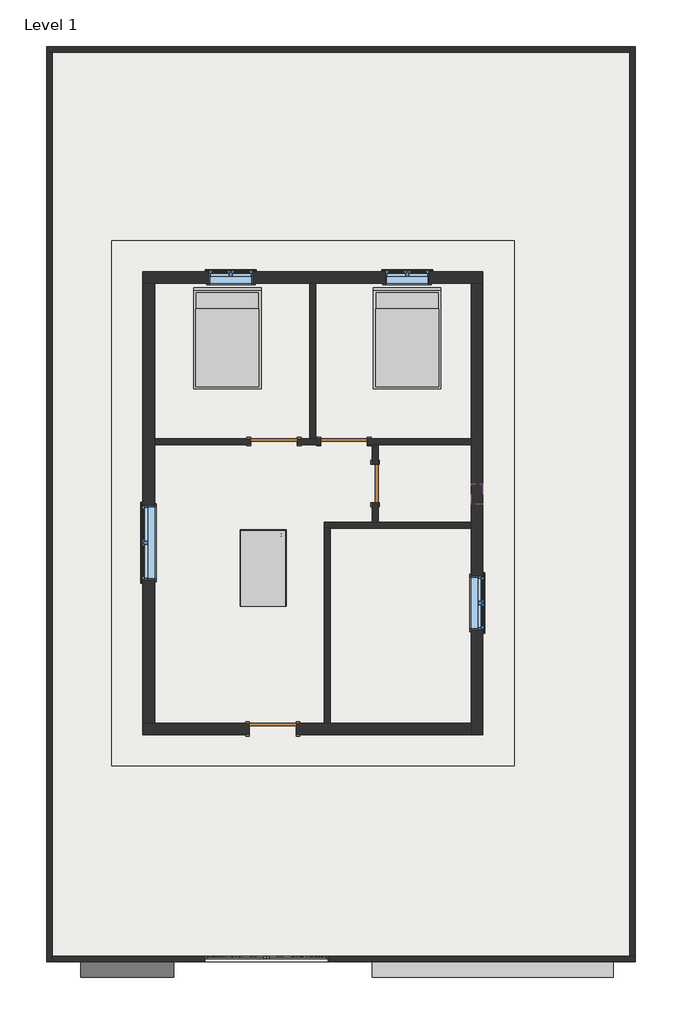
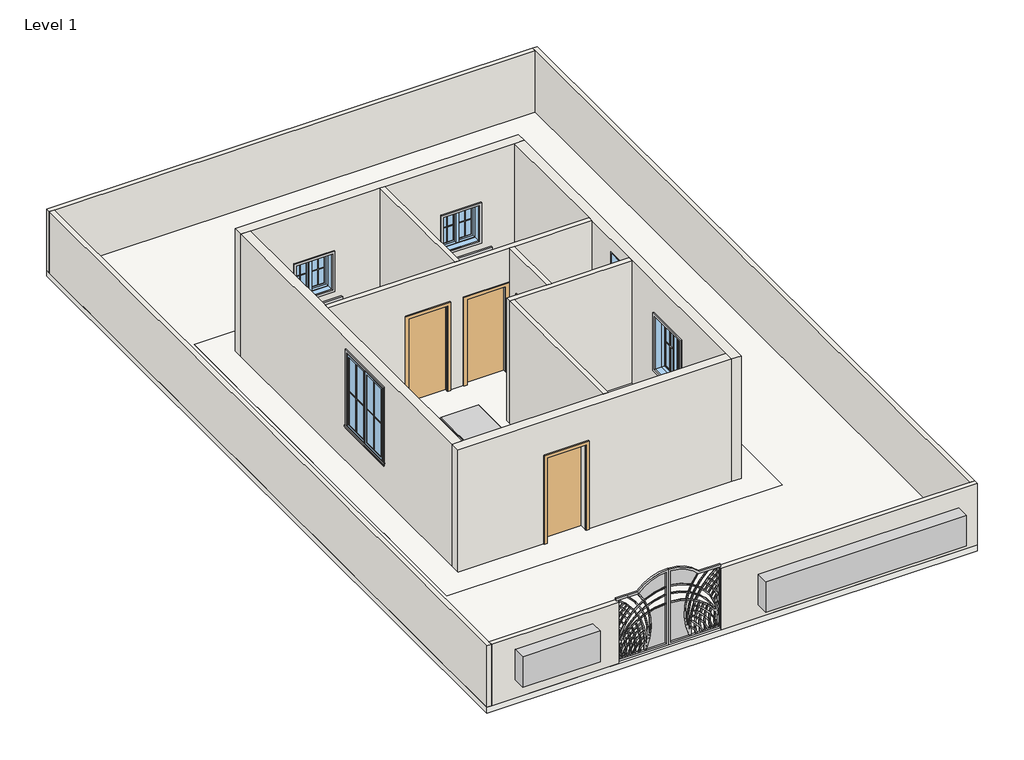
# One storey, incomplete: 18 proxies, 14 walls, 5 windows, 4 doors, 3 furniture elements, 2 slabs.
"""IFC4 building model written with IfcOpenShell, lengths in millimetres."""

from ifc_helpers import new_model, si_unit, frame, origin, origin_with_axes, place, context, project, spatial, polyline, outline, extrude, faceted_brep, transform, mapped, element, save
from components import generic_models_6bc30956, generic_models_2_generic_models_2_082925ae, muntin_pattern_2x2_muntin_pattern_2x2_b3fe6957, muntin_pattern_2x2_muntin_pattern_2x2_3e0ecaf2, muntin_pattern_2x2_muntin_pattern_2x2_bff912c5, muntin_pattern_2x2_muntin_pattern_2x2_c2194282, muntin_pattern_2x2_muntin_pattern_2x2_88bf7f41, muntin_pattern_2x2_muntin_pattern_2x2_3dfd0a47, trim_window_exterior_flat_with_sill_41619996, trim_window_exterior_flat_with_sill_e04b3088, trim_window_exterior_flat_with_sill_4930676f, trim_window_interior_flat_picture_frame_51c85655, trim_window_interior_flat_picture_frame_2a7685fe, trim_window_interior_flat_picture_frame_dd064338, door_f2b275c1, door_e5f9f3c4, door_305aa2a5, door_0ca8825f, bed_17739_bed_17739_15c61121, dining_table_14755_dining_table_14755_d89cb775, window_aa618e30, window_339605e1, window_c95ebb39, window_9ac97e1a

model = new_model("IFC4")

# Units and contexts
model_context = context("Model", 3, world=origin())
ifc_project = project(units=[si_unit("LENGTHUNIT", "METRE", prefix="MILLI")], contexts=[model_context])

# Site, building, storey
site = spatial("IfcSite", under=ifc_project)
building = spatial("IfcBuilding", under=site)
storey = spatial("IfcBuildingStorey", under=building, Name="Level 1", Elevation=0.0)

# Proxies
placement = place(None, origin())
generic_models_shape = generic_models_6bc30956(model_context)
element("IfcBuildingElementProxy", 1, Name="Generic Models", at=placement, inside=storey, context=model_context, shape_type="MappedRepresentation", body=[
    mapped(generic_models_shape, transform((-2169.6415084, -8339.9599223, 0.0), x_axis=(1.0, 0.0, 0.0), y_axis=(0.0, 1.0, 0.0), z_axis=(0.0, 0.0, 1.0))),
])
generic_models_2_generic_models_2_shape = generic_models_2_generic_models_2_082925ae(model_context)
element("IfcBuildingElementProxy", 2, Name="Generic Models 2 : Generic Models 2", ObjectType="Generic Models 2 : Generic Models 2", at=placement, inside=storey, context=model_context, shape_type="MappedRepresentation", body=[
    mapped(generic_models_2_generic_models_2_shape, transform((0.0, 0.0, 0.0), x_axis=(1.0, 0.0, 0.0), y_axis=(0.0, 1.0, 0.0), z_axis=(0.0, 0.0, 1.0))),
])
muntin_pattern_2x2_muntin_pattern_2x2_shape = muntin_pattern_2x2_muntin_pattern_2x2_b3fe6957(model_context)
element("IfcBuildingElementProxy", 3, Name="Muntin Pattern_2x2 : Muntin Pattern_2x2", ObjectType="Muntin Pattern_2x2 : Muntin Pattern_2x2", at=placement, inside=storey, context=model_context, shape_type="MappedRepresentation", body=[
    mapped(muntin_pattern_2x2_muntin_pattern_2x2_shape, transform((-3079.2790084, 5068.9185985, 984.25), x_axis=(1.0, 0.0, 0.0), y_axis=(0.0, 1.0, 0.0), z_axis=(0.0, 0.0, 1.0))),
])
element("IfcBuildingElementProxy", 4, Name="Muntin Pattern_2x2 : Muntin Pattern_2x2", ObjectType="Muntin Pattern_2x2 : Muntin Pattern_2x2", at=placement, inside=storey, context=model_context, shape_type="MappedRepresentation", body=[
    mapped(muntin_pattern_2x2_muntin_pattern_2x2_shape, transform((378.2959916, 5068.9185985, 984.25), x_axis=(1.0, 0.0, 0.0), y_axis=(0.0, 1.0, 0.0), z_axis=(0.0, 0.0, 1.0))),
])
muntin_pattern_2x2_muntin_pattern_2x2_2_shape = muntin_pattern_2x2_muntin_pattern_2x2_3e0ecaf2(model_context)
element("IfcBuildingElementProxy", 5, Name="Muntin Pattern_2x2 : Muntin Pattern_2x2", ObjectType="Muntin Pattern_2x2 : Muntin Pattern_2x2", at=placement, inside=storey, context=model_context, shape_type="MappedRepresentation", body=[
    mapped(muntin_pattern_2x2_muntin_pattern_2x2_2_shape, transform((-2650.6540084, 5068.9185985, 984.25), x_axis=(-1.0, 0.0, 0.0), y_axis=(0.0, -1.0, 0.0), z_axis=(0.0, 0.0, 1.0))),
])
element("IfcBuildingElementProxy", 6, Name="Muntin Pattern_2x2 : Muntin Pattern_2x2", ObjectType="Muntin Pattern_2x2 : Muntin Pattern_2x2", at=placement, inside=storey, context=model_context, shape_type="MappedRepresentation", body=[
    mapped(muntin_pattern_2x2_muntin_pattern_2x2_2_shape, transform((806.9209916, 5068.9185985, 984.25), x_axis=(-1.0, 0.0, 0.0), y_axis=(0.0, -1.0, 0.0), z_axis=(0.0, 0.0, 1.0))),
])
muntin_pattern_2x2_muntin_pattern_2x2_3_shape = muntin_pattern_2x2_muntin_pattern_2x2_bff912c5(model_context)
element("IfcBuildingElementProxy", 7, Name="Muntin Pattern_2x2 : Muntin Pattern_2x2", ObjectType="Muntin Pattern_2x2 : Muntin Pattern_2x2", at=placement, inside=storey, context=model_context, shape_type="MappedRepresentation", body=[
    mapped(muntin_pattern_2x2_muntin_pattern_2x2_3_shape, transform((-4579.4665084, -596.8689015, 984.25), x_axis=(0.0, 1.0, 0.0), y_axis=(-1.0, 0.0, 0.0), z_axis=(0.0, 0.0, 1.0))),
])
muntin_pattern_2x2_muntin_pattern_2x2_4_shape = muntin_pattern_2x2_muntin_pattern_2x2_c2194282(model_context)
element("IfcBuildingElementProxy", 8, Name="Muntin Pattern_2x2 : Muntin Pattern_2x2", ObjectType="Muntin Pattern_2x2 : Muntin Pattern_2x2", at=placement, inside=storey, context=model_context, shape_type="MappedRepresentation", body=[
    mapped(muntin_pattern_2x2_muntin_pattern_2x2_4_shape, transform((-4579.4665084, 123.8560985, 984.25), x_axis=(0.0, -1.0, 0.0), y_axis=(1.0, 0.0, 0.0), z_axis=(0.0, 0.0, 1.0))),
])
muntin_pattern_2x2_muntin_pattern_2x2_5_shape = muntin_pattern_2x2_muntin_pattern_2x2_88bf7f41(model_context)
element("IfcBuildingElementProxy", 9, Name="Muntin Pattern_2x2 : Muntin Pattern_2x2", ObjectType="Muntin Pattern_2x2 : Muntin Pattern_2x2", at=placement, inside=storey, context=model_context, shape_type="MappedRepresentation", body=[
    mapped(muntin_pattern_2x2_muntin_pattern_2x2_5_shape, transform((2068.9834916, -1158.8439015, 984.25), x_axis=(0.0, -1.0, 0.0), y_axis=(1.0, 0.0, 0.0), z_axis=(0.0, 0.0, 1.0))),
])
muntin_pattern_2x2_muntin_pattern_2x2_6_shape = muntin_pattern_2x2_muntin_pattern_2x2_3dfd0a47(model_context)
element("IfcBuildingElementProxy", 10, Name="Muntin Pattern_2x2 : Muntin Pattern_2x2", ObjectType="Muntin Pattern_2x2 : Muntin Pattern_2x2", at=placement, inside=storey, context=model_context, shape_type="MappedRepresentation", body=[
    mapped(muntin_pattern_2x2_muntin_pattern_2x2_6_shape, transform((2068.9834916, -1676.3689015, 984.25), x_axis=(0.0, 1.0, 0.0), y_axis=(-1.0, 0.0, 0.0), z_axis=(0.0, 0.0, 1.0))),
])
trim_window_exterior_flat_with_sill_shape = trim_window_exterior_flat_with_sill_41619996(model_context)
element("IfcBuildingElementProxy", 11, Name="Trim-Window-Exterior-Flat : with Sill", ObjectType="Trim-Window-Exterior-Flat : with Sill", at=placement, inside=storey, context=model_context, shape_type="MappedRepresentation", body=[
    mapped(trim_window_exterior_flat_with_sill_shape, transform((-2864.9665084, 5078.4435985, 1828.8), x_axis=(-1.0, 0.0, 0.0), y_axis=(0.0, 0.0, 1.0), z_axis=(0.0, 1.0, 0.0))),
])
element("IfcBuildingElementProxy", 12, Name="Trim-Window-Exterior-Flat : with Sill", ObjectType="Trim-Window-Exterior-Flat : with Sill", at=placement, inside=storey, context=model_context, shape_type="MappedRepresentation", body=[
    mapped(trim_window_exterior_flat_with_sill_shape, transform((592.6084916, 5078.4435985, 1828.8), x_axis=(-1.0, 0.0, 0.0), y_axis=(0.0, 0.0, 1.0), z_axis=(0.0, 1.0, 0.0))),
])
trim_window_exterior_flat_with_sill_2_shape = trim_window_exterior_flat_with_sill_e04b3088(model_context)
element("IfcBuildingElementProxy", 13, Name="Trim-Window-Exterior-Flat : with Sill", ObjectType="Trim-Window-Exterior-Flat : with Sill", at=placement, inside=storey, context=model_context, shape_type="MappedRepresentation", body=[
    mapped(trim_window_exterior_flat_with_sill_2_shape, transform((-4588.9915084, -236.5064015, 2743.2), x_axis=(0.0, -1.0, 0.0), y_axis=(0.0, 0.0, 1.0), z_axis=(-1.0, 0.0, 0.0))),
])
trim_window_exterior_flat_with_sill_3_shape = trim_window_exterior_flat_with_sill_4930676f(model_context)
element("IfcBuildingElementProxy", 14, Name="Trim-Window-Exterior-Flat : with Sill", ObjectType="Trim-Window-Exterior-Flat : with Sill", at=placement, inside=storey, context=model_context, shape_type="MappedRepresentation", body=[
    mapped(trim_window_exterior_flat_with_sill_3_shape, transform((2078.5084916, -1417.6064015, 2260.6), x_axis=(0.0, 1.0, 0.0), y_axis=(0.0, 0.0, 1.0), z_axis=(1.0, 0.0, 0.0))),
])
trim_window_interior_flat_picture_frame_shape = trim_window_interior_flat_picture_frame_51c85655(model_context)
element("IfcBuildingElementProxy", 15, Name="Trim-Window-Interior-Flat : Picture Frame", ObjectType="Trim-Window-Interior-Flat : Picture Frame", at=placement, inside=storey, context=model_context, shape_type="MappedRepresentation", body=[
    mapped(trim_window_interior_flat_picture_frame_shape, transform((-2864.9665084, 4849.8435985, 1828.8), x_axis=(1.0, 0.0, 0.0), y_axis=(0.0, 0.0, 1.0), z_axis=(0.0, -1.0, 0.0))),
])
element("IfcBuildingElementProxy", 16, Name="Trim-Window-Interior-Flat : Picture Frame", ObjectType="Trim-Window-Interior-Flat : Picture Frame", at=placement, inside=storey, context=model_context, shape_type="MappedRepresentation", body=[
    mapped(trim_window_interior_flat_picture_frame_shape, transform((592.6084916, 4849.8435985, 1828.8), x_axis=(1.0, 0.0, 0.0), y_axis=(0.0, 0.0, 1.0), z_axis=(0.0, -1.0, 0.0))),
])
trim_window_interior_flat_picture_frame_2_shape = trim_window_interior_flat_picture_frame_2a7685fe(model_context)
element("IfcBuildingElementProxy", 17, Name="Trim-Window-Interior-Flat : Picture Frame", ObjectType="Trim-Window-Interior-Flat : Picture Frame", at=placement, inside=storey, context=model_context, shape_type="MappedRepresentation", body=[
    mapped(trim_window_interior_flat_picture_frame_2_shape, transform((-4360.3915084, -236.5064015, 2743.2), x_axis=(0.0, 1.0, 0.0), y_axis=(0.0, 0.0, 1.0), z_axis=(1.0, 0.0, 0.0))),
])
trim_window_interior_flat_picture_frame_3_shape = trim_window_interior_flat_picture_frame_dd064338(model_context)
element("IfcBuildingElementProxy", 18, Name="Trim-Window-Interior-Flat : Picture Frame", ObjectType="Trim-Window-Interior-Flat : Picture Frame", at=placement, inside=storey, context=model_context, shape_type="MappedRepresentation", body=[
    mapped(trim_window_interior_flat_picture_frame_3_shape, transform((1849.9084916, -1417.6064015, 2260.6), x_axis=(0.0, -1.0, 0.0), y_axis=(0.0, 0.0, 1.0), z_axis=(-1.0, 0.0, 0.0))),
])

# Doors
door_shape = door_f2b275c1(model_context)
element("IfcDoor", 19, ObjectType="Single-Flush : 30\" x 80\"", at=placement, inside=storey, context=model_context, shape_type="MappedRepresentation", body=[
    mapped(door_shape, transform((-36.0415084, 925.5435985, 0.0), x_axis=(0.0, 1.0, 0.0), y_axis=(-1.0, 0.0, 0.0), z_axis=(0.0, 0.0, 1.0))),
])
door_2_shape = door_e5f9f3c4(model_context)
element("IfcDoor", 20, ObjectType="Single-Flush : 36\" x 84\"", at=placement, inside=storey, context=model_context, shape_type="MappedRepresentation", body=[
    mapped(door_2_shape, transform((-2017.2415084, 1744.6935985, 0.0), x_axis=(1.0, 0.0, 0.0), y_axis=(0.0, 1.0, 0.0), z_axis=(0.0, 0.0, 1.0))),
])
door_3_shape = door_305aa2a5(model_context)
element("IfcDoor", 21, ObjectType="Single-Flush : 36\" x 84\"", at=placement, inside=storey, context=model_context, shape_type="MappedRepresentation", body=[
    mapped(door_3_shape, transform((-645.6415084, 1744.6935985, 0.0), x_axis=(-1.0, 0.0, 0.0), y_axis=(0.0, -1.0, 0.0), z_axis=(0.0, 0.0, 1.0))),
])
door_4_shape = door_0ca8825f(model_context)
element("IfcDoor", 22, ObjectType="Single-Flush : 36\" x 84\"", at=placement, inside=storey, context=model_context, shape_type="MappedRepresentation", body=[
    mapped(door_4_shape, transform((-2042.6415084, -3887.7564015, 0.0), x_axis=(1.0, 0.0, 0.0), y_axis=(0.0, 1.0, 0.0), z_axis=(0.0, 0.0, 1.0))),
])

# Furniture
bed_17739_bed_17739_shape = bed_17739_bed_17739_15c61121(model_context)
element("IfcFurniture", 23, ObjectType="Bed_17739 : Bed_17739", at=placement, inside=storey, context=model_context, shape_type="MappedRepresentation", body=[
    mapped(bed_17739_bed_17739_shape, transform((-2931.6415084, 3744.9435985, 0.0), x_axis=(1.0, 0.0, 0.0), y_axis=(0.0, 1.0, 0.0), z_axis=(0.0, 0.0, 1.0))),
])
element("IfcFurniture", 24, ObjectType="Bed_17739 : Bed_17739", at=placement, inside=storey, context=model_context, shape_type="MappedRepresentation", body=[
    mapped(bed_17739_bed_17739_shape, transform((592.6084916, 3744.9435985, 0.0), x_axis=(1.0, 0.0, 0.0), y_axis=(0.0, 1.0, 0.0), z_axis=(0.0, 0.0, 1.0))),
])
dining_table_14755_dining_table_14755_shape = dining_table_14755_dining_table_14755_d89cb775(model_context)
element("IfcFurniture", 25, ObjectType="Dining_table_14755 : Dining_table_14755", at=placement, inside=storey, context=model_context, shape_type="MappedRepresentation", body=[
    mapped(dining_table_14755_dining_table_14755_shape, transform((-1781.6222109, -1485.4350296, 0.0), x_axis=(0.0, 1.0, 0.0), y_axis=(-1.0, 0.0, 0.0), z_axis=(0.0, 0.0, 1.0))),
])

# Slabs
element("IfcSlab", 26, ObjectType="Generic - 12\"", at=placement, inside=storey, context=model_context, shape_type="SweptSolid", body=[
    extrude(outline(polyline([(5067.1792532, 9490.8400777), (5067.1792532, -8454.2599223), (-6477.1207468, -8454.2599223), (-6477.1207468, 9490.8400777), (5067.1792532, 9490.8400777)])), frame((0.0, 0.0, -152.4), z_axis=(0.0, 0.0, 1.0), x_axis=(1.0, 0.0, 0.0)), (0.0, 0.0, 1.0), 152.4),
])
element("IfcSlab", 27, ObjectType="Generic - 12\"", at=placement, inside=storey, context=model_context, shape_type="SweptSolid", body=[
    extrude(outline(polyline([(2688.1084916, 5688.0435985), (2688.1084916, -4611.6564015), (-5198.5915084, -4611.6564015), (-5198.5915084, 5688.0435985), (2688.1084916, 5688.0435985)])), frame((0.0, 0.0, -152.4), z_axis=(0.0, 0.0, 1.0), x_axis=(1.0, 0.0, 0.0)), (0.0, 0.0, 1.0), 152.4),
])

# Walls
element("IfcWall", 28, ObjectType="WALL4.5\"", at=placement, inside=storey, context=model_context, shape_type="Brep", body=[
    faceted_brep([(-1560.0415084, 1687.5435985, 0.0), (-1102.8415084, 1687.5435985, 0.0), (-1102.8415084, 1687.5435985, 2133.6), (-188.4415084, 1687.5435985, 2133.6), (-188.4415084, 1687.5435985, 0.0), (-93.1915084, 1687.5435985, 0.0), (21.1084916, 1687.5435985, 0.0), (1849.9084916, 1687.5435985, 0.0), (1849.9084916, 1687.5435985, 3048.0), (21.1084916, 1687.5435985, 3048.0), (-93.1915084, 1687.5435985, 3048.0), (-4360.3915084, 1687.5435985, 3048.0), (-4360.3915084, 1687.5435985, 0.0), (-2474.4415084, 1687.5435985, 0.0), (-2474.4415084, 1687.5435985, 2133.6), (-1560.0415084, 1687.5435985, 2133.6), (-1102.8415084, 1801.8435985, 2133.6), (-1102.8415084, 1801.8435985, 0.0), (-1198.0915084, 1801.8435985, 0.0), (-1312.3915084, 1801.8435985, 0.0), (-1560.0415084, 1801.8435985, 0.0), (-1560.0415084, 1801.8435985, 2133.6), (-2474.4415084, 1801.8435985, 2133.6), (-2474.4415084, 1801.8435985, 0.0), (-4360.3915084, 1801.8435985, 0.0), (-4360.3915084, 1801.8435985, 3048.0), (-1312.3915084, 1801.8435985, 3048.0), (-1198.0915084, 1801.8435985, 3048.0), (1849.9084916, 1801.8435985, 3048.0), (1849.9084916, 1801.8435985, 0.0), (-188.4415084, 1801.8435985, 0.0), (-188.4415084, 1801.8435985, 2133.6)], [[[0, 1, 2, 3, 4, 5, 6, 7, 8, 9, 10, 11, 12, 13, 14, 15]], [[16, 17, 18, 19, 20, 21, 22, 23, 24, 25, 26, 27, 28, 29, 30, 31]], [[13, 12, 24, 23]], [[30, 29, 7, 6, 5, 4]], [[20, 19, 18, 17, 1, 0]], [[8, 7, 29, 28]], [[12, 11, 25, 24]], [[21, 20, 0, 15]], [[22, 21, 15, 14]], [[23, 22, 14, 13]], [[2, 1, 17, 16]], [[3, 2, 16, 31]], [[4, 3, 31, 30]], [[11, 10, 9, 8, 28, 27, 26, 25]]]),
])
element("IfcWall", 29, ObjectType="WALL4.5\"", at=placement, inside=storey, context=model_context, shape_type="SweptSolid", body=[
    extrude(outline(polyline([(-1312.3915084, 1801.8435985), (-1312.3915084, 4849.8435985), (-1198.0915084, 4849.8435985), (-1198.0915084, 1801.8435985), (-1312.3915084, 1801.8435985)])), origin_with_axes(), (0.0, 0.0, 1.0), 3048.0),
])
element("IfcWall", 30, ObjectType="WALL4.5\"", at=placement, inside=storey, context=model_context, shape_type="SweptSolid", body=[
    extrude(outline(polyline([(1687.5435985, 0.0), (1306.5435985, 0.0), (1306.5435985, 2032.0), (544.5435985, 2032.0), (544.5435985, 0.0), (163.5435985, 0.0), (163.5435985, 3048.0), (1687.5435985, 3048.0), (1687.5435985, 0.0)])), frame((-93.1915084, 0.0, 0.0), z_axis=(1.0, 0.0, 0.0), x_axis=(0.0, 1.0, 0.0)), (0.0, 0.0, 1.0), 114.3),
])
element("IfcWall", 31, ObjectType="WALL4.5\"", at=placement, inside=storey, context=model_context, shape_type="Brep", body=[
    faceted_brep([(1849.9084916, 163.5435985, 0.0), (21.1084916, 163.5435985, 0.0), (-93.1915084, 163.5435985, 0.0), (-1032.9915084, 163.5435985, 0.0), (-1032.9915084, 163.5435985, 3048.0), (-93.1915084, 163.5435985, 3048.0), (21.1084916, 163.5435985, 3048.0), (1849.9084916, 163.5435985, 3048.0), (1849.9084916, 49.2435985, 0.0), (1849.9084916, 49.2435985, 3048.0), (-918.6915084, 49.2435985, 3048.0), (-1032.9915084, 49.2435985, 3048.0), (-1032.9915084, 49.2435985, 0.0), (-918.6915084, 49.2435985, 0.0)], [[[0, 1, 2, 3, 4, 5, 6, 7]], [[8, 9, 10, 11, 12, 13]], [[3, 2, 1, 0, 8, 13, 12]], [[0, 7, 9, 8]], [[4, 3, 12, 11]], [[7, 6, 5, 4, 11, 10, 9]]]),
])
element("IfcWall", 32, ObjectType="WALL4.5\"", at=placement, inside=storey, context=model_context, shape_type="SweptSolid", body=[
    extrude(outline(polyline([(-1032.9915084, -3773.4564015), (-1032.9915084, 49.2435985), (-918.6915084, 49.2435985), (-918.6915084, -3773.4564015), (-1032.9915084, -3773.4564015)])), origin_with_axes(), (0.0, 0.0, 1.0), 3048.0),
])
element("IfcWall", 33, ObjectType="WALL4.5\"", at=placement, inside=storey, context=model_context, shape_type="Brep", body=[
    faceted_brep([(-6477.1207468, 9376.5400777, 0.0), (-6362.8207468, 9376.5400777, 0.0), (4952.8792532, 9376.5400777, 0.0), (4952.8792532, 9376.5400777, 1524.0), (-6362.8207468, 9376.5400777, 1524.0), (-6477.1207468, 9376.5400777, 1524.0), (-6477.1207468, 9490.8400777, 0.0), (-6477.1207468, 9490.8400777, 1524.0), (4952.8792532, 9490.8400777, 1524.0), (4952.8792532, 9490.8400777, 0.0)], [[[0, 1, 2, 3, 4, 5]], [[6, 7, 8, 9]], [[2, 1, 0, 6, 9]], [[5, 4, 3, 8, 7]], [[0, 5, 7, 6]], [[3, 2, 9, 8]]]),
])
element("IfcWall", 34, ObjectType="WALL4.5\"", at=placement, inside=storey, context=model_context, shape_type="Brep", body=[
    faceted_brep([(-6362.8207468, -8454.2599223, 0.0), (-6362.8207468, -8339.9599223, 0.0), (-6362.8207468, 9376.5400777, 0.0), (-6362.8207468, 9376.5400777, 1524.0), (-6362.8207468, -8339.9599223, 1524.0), (-6362.8207468, -8454.2599223, 1524.0), (-6477.1207468, -8454.2599223, 0.0), (-6477.1207468, -8454.2599223, 1524.0), (-6477.1207468, 9376.5400777, 1524.0), (-6477.1207468, 9376.5400777, 0.0)], [[[0, 1, 2, 3, 4, 5]], [[6, 7, 8, 9]], [[2, 1, 0, 6, 9]], [[5, 4, 3, 8, 7]], [[0, 5, 7, 6]], [[3, 2, 9, 8]]]),
])
element("IfcWall", 35, ObjectType="WALL4.5\"", at=placement, inside=storey, context=model_context, shape_type="Brep", body=[
    faceted_brep([(5067.1792532, -8339.9599223, 0.0), (4952.8792532, -8339.9599223, 0.0), (-958.9707468, -8339.9599223, 0.0), (-958.9707468, -8339.9599223, 1524.0), (4952.8792532, -8339.9599223, 1524.0), (5067.1792532, -8339.9599223, 1524.0), (5067.1792532, -8454.2599223, 0.0), (5067.1792532, -8454.2599223, 1524.0), (-958.9707468, -8454.2599223, 1524.0), (-958.9707468, -8454.2599223, 0.0)], [[[0, 1, 2, 3, 4, 5]], [[6, 7, 8, 9]], [[2, 1, 0, 6, 9]], [[3, 2, 9, 8]], [[5, 4, 3, 8, 7]], [[0, 5, 7, 6]]]),
])
element("IfcWall", 36, ObjectType="WALL4.5\"", at=placement, inside=storey, context=model_context, shape_type="Brep", body=[
    faceted_brep([(4952.8792532, 9490.8400777, 0.0), (4952.8792532, 9376.5400777, 0.0), (4952.8792532, -8339.9599223, 0.0), (4952.8792532, -8339.9599223, 1524.0), (4952.8792532, 9376.5400777, 1524.0), (4952.8792532, 9490.8400777, 1524.0), (5067.1792532, 9490.8400777, 0.0), (5067.1792532, 9490.8400777, 1524.0), (5067.1792532, -8339.9599223, 1524.0), (5067.1792532, -8339.9599223, 0.0)], [[[0, 1, 2, 3, 4, 5]], [[6, 7, 8, 9]], [[2, 1, 0, 6, 9]], [[5, 4, 3, 8, 7]], [[0, 5, 7, 6]], [[3, 2, 9, 8]]]),
])
element("IfcWall", 37, ObjectType="WALL4.5\"", at=placement, inside=storey, context=model_context, shape_type="SweptSolid", body=[
    extrude(outline(polyline([(-6362.8207468, -8339.9599223), (-3371.9707468, -8339.9599223), (-3371.9707468, -8454.2599223), (-6362.8207468, -8454.2599223), (-6362.8207468, -8339.9599223)])), origin_with_axes(), (0.0, 0.0, 1.0), 1524.0),
])
element("IfcWall", 38, ObjectType="WALL9\"", at=placement, inside=storey, context=model_context, shape_type="Brep", body=[
    faceted_brep([(-4588.9915084, 4849.8435985, 0.0), (-4360.3915084, 4849.8435985, 0.0), (-1312.3915084, 4849.8435985, 0.0), (-1198.0915084, 4849.8435985, 0.0), (1849.9084916, 4849.8435985, 0.0), (2078.5084916, 4849.8435985, 0.0), (2078.5084916, 4849.8435985, 3048.0), (1849.9084916, 4849.8435985, 3048.0), (-1198.0915084, 4849.8435985, 3048.0), (-1312.3915084, 4849.8435985, 3048.0), (-4360.3915084, 4849.8435985, 3048.0), (-4588.9915084, 4849.8435985, 3048.0), (-2433.1665084, 4849.8435985, 1828.8), (-2433.1665084, 4849.8435985, 914.4), (-3296.7665084, 4849.8435985, 914.4), (-3296.7665084, 4849.8435985, 1828.8), (1024.4084916, 4849.8435985, 1828.8), (1024.4084916, 4849.8435985, 914.4), (160.8084916, 4849.8435985, 914.4), (160.8084916, 4849.8435985, 1828.8), (-4588.9915084, 5078.4435985, 0.0), (-4588.9915084, 5078.4435985, 3048.0), (2078.5084916, 5078.4435985, 3048.0), (2078.5084916, 5078.4435985, 0.0), (-2433.1665084, 5078.4435985, 1828.8), (-3296.7665084, 5078.4435985, 1828.8), (-3296.7665084, 5078.4435985, 914.4), (-2433.1665084, 5078.4435985, 914.4), (1024.4084916, 5078.4435985, 1828.8), (160.8084916, 5078.4435985, 1828.8), (160.8084916, 5078.4435985, 914.4), (1024.4084916, 5078.4435985, 914.4)], [[[0, 1, 2, 3, 4, 5, 6, 7, 8, 9, 10, 11], [12, 13, 14, 15], [16, 17, 18, 19]], [[20, 21, 22, 23], [24, 25, 26, 27], [28, 29, 30, 31]], [[5, 4, 3, 2, 1, 0, 20, 23]], [[6, 5, 23, 22]], [[0, 11, 21, 20]], [[13, 12, 24, 27]], [[14, 13, 27, 26]], [[15, 14, 26, 25]], [[12, 15, 25, 24]], [[17, 16, 28, 31]], [[18, 17, 31, 30]], [[19, 18, 30, 29]], [[16, 19, 29, 28]], [[11, 10, 9, 8, 7, 6, 22, 21]]]),
])
element("IfcWall", 39, ObjectType="WALL9\"", at=placement, inside=storey, context=model_context, shape_type="Brep", body=[
    faceted_brep([(1849.9084916, 4849.8435985, 0.0), (1849.9084916, 1801.8435985, 0.0), (1849.9084916, 1687.5435985, 0.0), (1849.9084916, 163.5435985, 0.0), (1849.9084916, 49.2435985, 0.0), (1849.9084916, -3773.4564015, 0.0), (1849.9084916, -4002.0564015, 0.0), (1849.9084916, -4002.0564015, 3048.0), (1849.9084916, -3773.4564015, 3048.0), (1849.9084916, 49.2435985, 3048.0), (1849.9084916, 163.5435985, 3048.0), (1849.9084916, 1687.5435985, 3048.0), (1849.9084916, 1801.8435985, 3048.0), (1849.9084916, 4849.8435985, 3048.0), (1849.9084916, -1938.3064015, 2260.6), (1849.9084916, -1938.3064015, 914.4), (1849.9084916, -896.9064015, 914.4), (1849.9084916, -896.9064015, 2260.6), (1849.9084916, 512.7935985, 2743.2), (1849.9084916, 512.7935985, 2133.6), (1849.9084916, 919.1935985, 2133.6), (1849.9084916, 919.1935985, 2743.2), (2078.5084916, 4849.8435985, 0.0), (2078.5084916, 4849.8435985, 3048.0), (2078.5084916, -4002.0564015, 3048.0), (2078.5084916, -4002.0564015, 0.0), (2078.5084916, -1938.3064015, 2260.6), (2078.5084916, -896.9064015, 2260.6), (2078.5084916, -896.9064015, 914.4), (2078.5084916, -1938.3064015, 914.4), (2078.5084916, 512.7935985, 2743.2), (2078.5084916, 919.1935985, 2743.2), (2078.5084916, 919.1935985, 2133.6), (2078.5084916, 512.7935985, 2133.6)], [[[0, 1, 2, 3, 4, 5, 6, 7, 8, 9, 10, 11, 12, 13], [14, 15, 16, 17], [18, 19, 20, 21]], [[22, 23, 24, 25], [26, 27, 28, 29], [30, 31, 32, 33]], [[6, 5, 4, 3, 2, 1, 0, 22, 25]], [[0, 13, 23, 22]], [[7, 6, 25, 24]], [[15, 14, 26, 29]], [[16, 15, 29, 28]], [[17, 16, 28, 27]], [[14, 17, 27, 26]], [[19, 18, 30, 33]], [[20, 19, 33, 32]], [[21, 20, 32, 31]], [[18, 21, 31, 30]], [[13, 12, 11, 10, 9, 8, 7, 24, 23]]]),
])
element("IfcWall", 40, ObjectType="WALL9\"", at=placement, inside=storey, context=model_context, shape_type="Brep", body=[
    faceted_brep([(1849.9084916, -3773.4564015, 0.0), (-918.6915084, -3773.4564015, 0.0), (-1032.9915084, -3773.4564015, 0.0), (-1585.4415084, -3773.4564015, 0.0), (-1585.4415084, -3773.4564015, 2133.6), (-2499.8415084, -3773.4564015, 2133.6), (-2499.8415084, -3773.4564015, 0.0), (-4360.3915084, -3773.4564015, 0.0), (-4588.9915084, -3773.4564015, 0.0), (-4588.9915084, -3773.4564015, 3048.0), (-4360.3915084, -3773.4564015, 3048.0), (-1032.9915084, -3773.4564015, 3048.0), (-918.6915084, -3773.4564015, 3048.0), (1849.9084916, -3773.4564015, 3048.0), (-1585.4415084, -4002.0564015, 2133.6), (-1585.4415084, -4002.0564015, 0.0), (1849.9084916, -4002.0564015, 0.0), (1849.9084916, -4002.0564015, 3048.0), (-4588.9915084, -4002.0564015, 3048.0), (-4588.9915084, -4002.0564015, 0.0), (-2499.8415084, -4002.0564015, 0.0), (-2499.8415084, -4002.0564015, 2133.6)], [[[0, 1, 2, 3, 4, 5, 6, 7, 8, 9, 10, 11, 12, 13]], [[14, 15, 16, 17, 18, 19, 20, 21]], [[20, 19, 8, 7, 6]], [[16, 15, 3, 2, 1, 0]], [[0, 13, 17, 16]], [[9, 8, 19, 18]], [[4, 3, 15, 14]], [[5, 4, 14, 21]], [[6, 5, 21, 20]], [[13, 12, 11, 10, 9, 18, 17]]]),
])
element("IfcWall", 41, ObjectType="WALL9\"", at=placement, inside=storey, context=model_context, shape_type="Brep", body=[
    faceted_brep([(-4360.3915084, -3773.4564015, 0.0), (-4360.3915084, 1687.5435985, 0.0), (-4360.3915084, 1801.8435985, 0.0), (-4360.3915084, 4849.8435985, 0.0), (-4360.3915084, 4849.8435985, 3048.0), (-4360.3915084, 1801.8435985, 3048.0), (-4360.3915084, 1687.5435985, 3048.0), (-4360.3915084, -3773.4564015, 3048.0), (-4360.3915084, 487.3935985, 2743.2), (-4360.3915084, 487.3935985, 914.4), (-4360.3915084, -960.4064015, 914.4), (-4360.3915084, -960.4064015, 2743.2), (-4588.9915084, -3773.4564015, 0.0), (-4588.9915084, -3773.4564015, 3048.0), (-4588.9915084, 4849.8435985, 3048.0), (-4588.9915084, 4849.8435985, 0.0), (-4588.9915084, 487.3935985, 2743.2), (-4588.9915084, -960.4064015, 2743.2), (-4588.9915084, -960.4064015, 914.4), (-4588.9915084, 487.3935985, 914.4)], [[[0, 1, 2, 3, 4, 5, 6, 7], [8, 9, 10, 11]], [[12, 13, 14, 15], [16, 17, 18, 19]], [[3, 2, 1, 0, 12, 15]], [[0, 7, 13, 12]], [[4, 3, 15, 14]], [[9, 8, 16, 19]], [[10, 9, 19, 18]], [[11, 10, 18, 17]], [[8, 11, 17, 16]], [[7, 6, 5, 4, 14, 13]]]),
])

# Windows
window_shape = window_aa618e30(model_context)
element("IfcWindow", 42, ObjectType="Fixed : 16\" x 24\"", at=placement, inside=storey, context=model_context, shape_type="MappedRepresentation", body=[
    mapped(window_shape, transform((1964.2084916, 677.8935985, 1219.2), x_axis=(0.0, -1.0, 0.0), y_axis=(1.0, 0.0, 0.0), z_axis=(0.0, 0.0, 1.0))),
])
window_2_shape = window_339605e1(model_context)
element("IfcWindow", 43, ObjectType="Window-Casement-Double : 34\" x 36\"", at=placement, inside=storey, context=model_context, shape_type="MappedRepresentation", body=[
    mapped(window_2_shape, transform((-2864.9665084, 4964.1435985, 0.0), x_axis=(1.0, 0.0, 0.0), y_axis=(0.0, 1.0, 0.0), z_axis=(0.0, 0.0, 1.0))),
])
element("IfcWindow", 44, ObjectType="Window-Casement-Double : 34\" x 36\"", at=placement, inside=storey, context=model_context, shape_type="MappedRepresentation", body=[
    mapped(window_2_shape, transform((592.6084916, 4964.1435985, 0.0), x_axis=(1.0, 0.0, 0.0), y_axis=(0.0, 1.0, 0.0), z_axis=(0.0, 0.0, 1.0))),
])
window_3_shape = window_c95ebb39(model_context)
element("IfcWindow", 45, ObjectType="Window-Casement-Double : 41\" x 53\"", at=placement, inside=storey, context=model_context, shape_type="MappedRepresentation", body=[
    mapped(window_3_shape, transform((1964.2084916, -1417.6064015, 0.0), x_axis=(0.0, -1.0, 0.0), y_axis=(1.0, 0.0, 0.0), z_axis=(0.0, 0.0, 1.0))),
])
window_4_shape = window_9ac97e1a(model_context)
element("IfcWindow", 46, ObjectType="Window-Casement-Double : 57\" x 72\"", at=placement, inside=storey, context=model_context, shape_type="MappedRepresentation", body=[
    mapped(window_4_shape, transform((-4474.6915084, -236.5064015, 0.0), x_axis=(0.0, 1.0, 0.0), y_axis=(-1.0, 0.0, 0.0), z_axis=(0.0, 0.0, 1.0))),
])

save(model, "model.ifc")

# Revit data of these elements
# Type
#   m.s. sheet = none
#   2" x2" pipe = none
#   1"x1"pipe = none
#   Default Elevation = 0
# Type "Muntin Pattern_2x2 : Muntin Pattern_2x2"
#   Width [instance default] = 4' - 0"
#   Thickness = 0' - 0 1/2"
#   Height [instance default] = 4' - 0"
#   Distance = 0' - 0 3/4"
#   Interior Material [instance default] = none
#   Exterior Material [instance default] = none
#   Default Elevation = 0
# Type "Trim-Window-Exterior-Flat : with Sill"
#   Trim Width = 0' - 2 1/4"
#   Trim Thickness_Picture Frame = 0' - 1 1/4"
#   Trim Thickness_with Sill = 0' - 0 3/4"
#   Sill Thickness = 0' - 1 1/4"
#   Opening Width [instance default] = 2' - 0"
#   Opening Height [instance default] = 3' - 0"
#   Default Elevation = 4' - 0"
#   Sill = yes
#   Picture Frame = no
#   Trim Material [instance default] = none
# Type "Trim-Window-Interior-Flat : Picture Frame"
#   Trim Thickness_Picture Frame = 0' - 1 1/4"
#   Trim Width = 0' - 2 1/4"
#   Trim Thickness_with Sill = 0' - 0 3/4"
#   Sill Thickness = 0' - 1 1/4"
#   Opening Width [instance default] = 2' - 0"
#   Opening Height [instance default] = 3' - 0"
#   Default Elevation = 4' - 0"
#   Sill = no
#   Picture Frame = yes
#   Trim Material [instance default] = none
# Type "Single-Flush : 30\" x 80\""
#   Type Mark = "5"
#   Construction Type Id = "MDOOR"
#   Assembly Code = "C1020"
#   Analytic Construction = "Metal"
#   Thickness = 0' - 2"
#   Heat Transfer Coefficient (U) = 0.651978 BTU/(h·ft²·°F)
#   Height = 6' - 8"
#   Trim Projection Ext = 0' - 1"
#   Trim Projection Int = 0' - 1"
#   Trim Width = 0' - 3"
#   Width = 2' - 6"
#   Define Thermal Properties by = 1
#   Define Thermal Properties by = 1
#   Door Material = Door - Panel
#   Frame Material = Door - Frame
#   Visual Light Transmittance = 0
#   Solar Heat Gain Coefficient = 0
#   Function = (empty or 0)
#   Wall Closure = (empty or 0)
# Type "Single-Flush : 36\" x 84\""
#   Type Mark = "1"
#   Construction Type Id = "MDOOR"
#   Assembly Code = "C1020"
#   Analytic Construction = "Metal"
#   Thickness = 0' - 2"
#   Heat Transfer Coefficient (U) = 0.651978 BTU/(h·ft²·°F)
#   Height = 7' - 0"
#   Trim Projection Ext = 0' - 1"
#   Trim Projection Int = 0' - 1"
#   Trim Width = 0' - 3"
#   Width = 3' - 0"
#   Define Thermal Properties by = 1
#   Define Thermal Properties by = 1
#   Door Material = Door - Panel
#   Frame Material = Door - Frame
#   Visual Light Transmittance = 0
#   Solar Heat Gain Coefficient = 0
#   Function = (empty or 0)
#   Wall Closure = (empty or 0)
# Type "Bed_17739 : Bed_17739"
#   Default Elevation = 0
# Type "Dining_table_14755 : Dining_table_14755"
#   Lengte [instance default] = 4' - 11.05512"
#   Breedte [instance default] = 2' - 11.43307"
#   Tafelblad = none
#   Poten = none
#   Default Elevation = 0
# Type "Generic - 12\""
#   Assembly Code = "B1010"
#   Function = 0
#   Layers, outside or top first: 0' - 6" no material (function 1)
# Type "WALL4.5\""
#   Assembly Code = "B2010"
#   Layers, outside or top first: 0' - 4 1/2" no material (function 1)
# Type "WALL9\""
#   Assembly Code = "B2010"
#   Layers, outside or top first: 0' - 9" no material (function 1)
# Type "Fixed : 16\" x 24\""
#   Type Mark = "4"
#   Construction Type Id = "GSP4R"
#   Assembly Code = "B2020100"
#   Analytic Construction = "1/8 in Pilkington single glazing"
#   Visual Light Transmittance = 0.9
#   Solar Heat Gain Coefficient = 0.78
#   Heat Transfer Coefficient (U) = 0.6496 BTU/(h·ft²·°F)
#   Height = 2' - 0"
#   Default Sill Height = 3' - 0"
#   Width = 1' - 4"
#   Window Inset = 0' - 0 3/4"
#   Define Thermal Properties by = 1
#   Define Thermal Properties by = 1
#   Glass Pane Material = Glass
#   Sash Material = Sash
#   Wall Closure = (empty or 0)
# Type "Window-Casement-Double : 34\" x 36\""
#   Type Mark = "14"
#   Fire Rating = "0.5h"
#   Assembly Code = "B2020100"
#   Analytic Construction = "Double glazing - domestic"
#   Frame Extension [instance default] = 0' - 0 1/4"
#   Window Inset [instance default] = 0' - 0"
#   Wall Thickness [instance default] = 0' - 6"
#   Interior Wall Closure [instance default] = 0' - 2 1/4"
#   Half Width = 1' - 5"
#   Visual Light Transmittance = 0.81
#   Thermal Resistance (R) = 1.8146 (h·ft²·°F)/BTU
#   Solar Heat Gain Coefficient = 0.76
#   Rough Width = 2' - 10 1/2"
#   Rough Height = 3' - 0 1/2"
#   Height = 3' - 0"
#   Heat Transfer Coefficient (U) = 0.5511 BTU/(h·ft²·°F)
#   Exterior Wall Closure [instance default] = 0' - 1 1/4"
#   Extension Jamb [instance default] = 0' - 2 1/4"
#   Default Sill Height = 3' - 0"
#   Width = 2' - 10"
#   Define Thermal Properties by = 0
#   Muntin Visibility = yes
#   Interior Trim Visibility [instance default] = yes
#   Exterior Trim Visibility [instance default] = yes
#   Extension Jamb Visibility [instance default] = yes
#   Interior Trim Material = Wood - Stained
#   Muntin Pattern = Muntin Pattern_2x2 : Muntin Pattern_2x2
#   Interior Trim = Trim-Window-Interior-Flat : Picture Frame
#   Interior Frame Material = Wood - Stained
#   Glass Panel Material = Glass
#   Exterior Trim Material = Clad - White
#   Exterior Trim = Trim-Window-Exterior-Flat : with Sill
#   Exterior Frame Material = Clad - White
#   Wall Closure = (empty or 0)
# Type "Window-Casement-Double : 41\" x 53\""
#   Type Mark = "15"
#   Fire Rating = "0.5h"
#   Assembly Code = "B2020100"
#   Analytic Construction = "Double glazing - domestic"
#   Frame Extension [instance default] = 0' - 0 1/4"
#   Window Inset [instance default] = 0' - 0"
#   Wall Thickness [instance default] = 0' - 6"
#   Interior Wall Closure [instance default] = 0' - 2 1/4"
#   Half Width = 1' - 8 1/2"
#   Visual Light Transmittance = 0.81
#   Thermal Resistance (R) = 1.8146 (h·ft²·°F)/BTU
#   Solar Heat Gain Coefficient = 0.76
#   Rough Width = 3' - 5 1/2"
#   Rough Height = 4' - 5 1/2"
#   Height = 4' - 5"
#   Heat Transfer Coefficient (U) = 0.5511 BTU/(h·ft²·°F)
#   Exterior Wall Closure [instance default] = 0' - 1 1/4"
#   Extension Jamb [instance default] = 0' - 2 1/4"
#   Default Sill Height = 3' - 0"
#   Width = 3' - 5"
#   Define Thermal Properties by = 0
#   Muntin Visibility = yes
#   Interior Trim Visibility [instance default] = yes
#   Exterior Trim Visibility [instance default] = yes
#   Extension Jamb Visibility [instance default] = yes
#   Interior Trim Material = Wood - Stained
#   Muntin Pattern = Muntin Pattern_2x2 : Muntin Pattern_2x2
#   Interior Trim = Trim-Window-Interior-Flat : Picture Frame
#   Interior Frame Material = Wood - Stained
#   Glass Panel Material = Glass
#   Exterior Trim Material = Clad - White
#   Exterior Trim = Trim-Window-Exterior-Flat : with Sill
#   Exterior Frame Material = Clad - White
#   Wall Closure = (empty or 0)
# Type "Window-Casement-Double : 57\" x 72\""
#   Type Mark = "17"
#   Fire Rating = "0.5h"
#   Assembly Code = "B2020100"
#   Analytic Construction = "Double glazing - domestic"
#   Frame Extension [instance default] = 0' - 0 1/4"
#   Window Inset [instance default] = 0' - 0"
#   Wall Thickness [instance default] = 0' - 6"
#   Interior Wall Closure [instance default] = 0' - 2 1/4"
#   Half Width = 2' - 4 1/2"
#   Visual Light Transmittance = 0.81
#   Thermal Resistance (R) = 1.8146 (h·ft²·°F)/BTU
#   Solar Heat Gain Coefficient = 0.76
#   Rough Width = 4' - 9 1/2"
#   Rough Height = 6' - 0 1/2"
#   Height = 6' - 0"
#   Heat Transfer Coefficient (U) = 0.5511 BTU/(h·ft²·°F)
#   Exterior Wall Closure [instance default] = 0' - 1 1/4"
#   Extension Jamb [instance default] = 0' - 2 1/4"
#   Default Sill Height = 3' - 0"
#   Width = 4' - 9"
#   Define Thermal Properties by = 0
#   Muntin Visibility = yes
#   Interior Trim Visibility [instance default] = yes
#   Exterior Trim Visibility [instance default] = yes
#   Extension Jamb Visibility [instance default] = yes
#   Interior Trim Material = Wood - Stained
#   Muntin Pattern = Muntin Pattern_2x2 : Muntin Pattern_2x2
#   Interior Trim = Trim-Window-Interior-Flat : Picture Frame
#   Interior Frame Material = Wood - Stained
#   Glass Panel Material = Glass
#   Exterior Trim Material = Clad - White
#   Exterior Trim = Trim-Window-Exterior-Flat : with Sill
#   Exterior Frame Material = Clad - White
#   Wall Closure = (empty or 0)
# Element 1 (IfcBuildingElementProxy)
#   Phase Created = New Construction
#   Materials on its faces: "r1"
# Element 2 (IfcBuildingElementProxy, "Generic Models 2 : Generic Models 2")
#   Phase Created = New Construction
#   Materials on its faces: "Carpet (1)"
# Elements 3, 4, 5, 6 (IfcBuildingElementProxy, "Muntin Pattern_2x2 : Muntin Pattern_2x2")
#   Width = 0' - 11 5/8"
#   Height = 2' - 6 1/2"
#   Interior Material = Wood - Stained
#   Exterior Material = Clad - White
#   Phase Created = New Construction
#   Materials on its faces: "Clad - White", "Wood - Stained"
# Elements 7, 8 (IfcBuildingElementProxy, "Muntin Pattern_2x2 : Muntin Pattern_2x2")
#   Width = 1' - 11 1/8"
#   Height = 5' - 6 1/2"
#   Interior Material = Wood - Stained
#   Exterior Material = Clad - White
#   Phase Created = New Construction
#   Materials on its faces: "Clad - White", "Wood - Stained"
# Elements 9, 10 (IfcBuildingElementProxy, "Muntin Pattern_2x2 : Muntin Pattern_2x2")
#   Width = 1' - 3 1/8"
#   Height = 3' - 11 1/2"
#   Interior Material = Wood - Stained
#   Exterior Material = Clad - White
#   Phase Created = New Construction
#   Materials on its faces: "Clad - White", "Wood - Stained"
# Elements 11, 12 (IfcBuildingElementProxy, "Trim-Window-Exterior-Flat : with Sill")
#   Opening Width = 2' - 10"
#   Opening Height = 3' - 0"
#   Trim Material = Clad - White
#   Phase Created = New Construction
#   Materials on its faces: "Clad - White"
# Element 13 (IfcBuildingElementProxy, "Trim-Window-Exterior-Flat : with Sill")
#   Opening Width = 4' - 9"
#   Opening Height = 6' - 0"
#   Trim Material = Clad - White
#   Phase Created = New Construction
#   Materials on its faces: "Clad - White"
# Element 14 (IfcBuildingElementProxy, "Trim-Window-Exterior-Flat : with Sill")
#   Opening Width = 3' - 5"
#   Opening Height = 4' - 5"
#   Trim Material = Clad - White
#   Phase Created = New Construction
#   Materials on its faces: "Clad - White"
# Elements 15, 16 (IfcBuildingElementProxy, "Trim-Window-Interior-Flat : Picture Frame")
#   Opening Width = 2' - 10"
#   Opening Height = 3' - 0"
#   Trim Material = Wood - Stained
#   Phase Created = New Construction
#   Materials on its faces: "Wood - Stained"
# Element 17 (IfcBuildingElementProxy, "Trim-Window-Interior-Flat : Picture Frame")
#   Opening Width = 4' - 9"
#   Opening Height = 6' - 0"
#   Trim Material = Wood - Stained
#   Phase Created = New Construction
#   Materials on its faces: "Wood - Stained"
# Element 18 (IfcBuildingElementProxy, "Trim-Window-Interior-Flat : Picture Frame")
#   Opening Width = 3' - 5"
#   Opening Height = 4' - 5"
#   Trim Material = Wood - Stained
#   Phase Created = New Construction
#   Materials on its faces: "Wood - Stained"
# Element 19 (IfcDoor, "Single-Flush : 30\" x 80\"")
#   Phase Created = New Construction
#   Materials on its faces: "Door - Frame", "Door - Panel"
# Elements 20, 21, 22 (IfcDoor, "Single-Flush : 36\" x 84\"")
#   Phase Created = New Construction
#   Materials on its faces: "Door - Frame", "Door - Panel"
# Elements 23, 24 (IfcFurniture, "Bed_17739 : Bed_17739")
#   Phase Created = New Construction
#   Materials on its faces: "legs", "sheets", "bed frame", "Blanket"
# Element 25 (IfcFurniture, "Dining_table_14755 : Dining_table_14755")
#   Lengte = 4' - 11.05512"
#   Breedte = 2' - 11.43307"
#   Phase Created = New Construction
# Elements 26, 27 (IfcSlab, "Generic - 12\"")
#   Height Offset From Level = 0' - 0"
#   Phase Created = New Construction
#   Materials on its faces: "Default Floor"
# Elements 28, 29, 30, 31, 32 (IfcWall, "WALL4.5\"")
#   Top Offset = 0' - 0"
#   Base Offset = 0' - 0"
#   Unconnected Height = 10' - 0"
#   wall height = 10' - 0"
#   Phase Created = New Construction
#   Base Constraint = Level 1
#   Materials on its faces: "Default Wall"
# Elements 33, 34, 35, 36, 37 (IfcWall, "WALL4.5\"")
#   Top Offset = 0' - 0"
#   Base Offset = 0' - 0"
#   Unconnected Height = 5' - 0"
#   wall height = 5' - 0"
#   Phase Created = New Construction
#   Base Constraint = Level 1
#   Materials on its faces: "Default Wall", "Clad - White"
# Elements 38, 39, 40, 41 (IfcWall, "WALL9\"")
#   Top Offset = 0' - 0"
#   Base Offset = 0' - 0"
#   Unconnected Height = 10' - 0"
#   wall height = 10' - 0"
#   Phase Created = New Construction
#   Base Constraint = Level 1
#   Materials on its faces: "Default Wall", "Wood Planks"
# Element 42 (IfcWindow, "Fixed : 16\" x 24\"")
#   Mark = "5"
#   Phase Created = New Construction
#   Materials on its faces: "Sash", "Glass"
# Element 43 (IfcWindow, "Window-Casement-Double : 34\" x 36\"")
#   Mark = "1"
#   Window Inset = 0' - 0"
#   Interior Wall Closure = 0' - 2 1/4"
#   Frame Extension = 0' - 0 1/4"
#   Exterior Wall Closure = 0' - 1 1/4"
#   Interior Trim Visibility = yes
#   Exterior Trim Visibility = yes
#   Phase Created = New Construction
#   Materials on its faces: "Wood - Stained", "Glass", "Clad - White"
# Element 44 (IfcWindow, "Window-Casement-Double : 34\" x 36\"")
#   Mark = "2"
#   Window Inset = 0' - 0"
#   Interior Wall Closure = 0' - 2 1/4"
#   Frame Extension = 0' - 0 1/4"
#   Exterior Wall Closure = 0' - 1 1/4"
#   Interior Trim Visibility = yes
#   Exterior Trim Visibility = yes
#   Phase Created = New Construction
#   Materials on its faces: "Wood - Stained", "Glass", "Clad - White"
# Element 45 (IfcWindow, "Window-Casement-Double : 41\" x 53\"")
#   Mark = "4"
#   Window Inset = 0' - 0"
#   Interior Wall Closure = 0' - 2 1/4"
#   Frame Extension = 0' - 0 1/4"
#   Exterior Wall Closure = 0' - 1 1/4"
#   Interior Trim Visibility = yes
#   Exterior Trim Visibility = yes
#   Phase Created = New Construction
#   Materials on its faces: "Wood - Stained", "Glass", "Clad - White"
# Element 46 (IfcWindow, "Window-Casement-Double : 57\" x 72\"")
#   Mark = "3"
#   Window Inset = 0' - 0"
#   Interior Wall Closure = 0' - 2 1/4"
#   Frame Extension = 0' - 0 1/4"
#   Exterior Wall Closure = 0' - 1 1/4"
#   Interior Trim Visibility = yes
#   Exterior Trim Visibility = yes
#   Phase Created = New Construction
#   Materials on its faces: "Wood - Stained", "Glass", "Clad - White"
# Materials
#   "Door - Panel": class "Wood", colour RGB 210 159 95, transparency 0, Cost = 0
#   "Door - Frame": colour RGB 118 70 51, transparency 0, Cost = 0
#   "Glass": class "Glass", colour RGB 0 128 192, transparency 0.75, Description = "Soda Lime Glass", Cost = 0
#   "Sash": class "Wood", colour RGB 224 178 126, transparency 0, Cost = 0
#   "Wood - Stained": class "Wood", colour RGB 224 178 126, transparency 0, Cost = 0
#   "Clad - White": class "Wood", colour RGB 242 242 238, transparency 0, Cost = 0
#   "r1": class "Generic", colour RGB 120 120 120, transparency 0, Cost = 0
#   "Carpet (1)": class "Carpet", colour RGB 124 80 67, transparency 0, Description = "Interior finish", Cost = 0
#   "legs": colour RGB 90 73 37, transparency 0, Cost = 0
#   "sheets": colour RGB 200 195 176, transparency 0, Cost = 0
#   "bed frame": colour RGB 90 73 37, transparency 0, Cost = 0
#   "Blanket": class "System", colour RGB 59 0 1, transparency 0, Cost = 0
#   "Default Floor": colour RGB 128 128 128, transparency 0, Cost = 0
#   "Default Wall": colour RGB 128 128 128, transparency 0, Cost = 0
#   "Wood Planks": class "Wood", colour RGB 193 160 115, transparency 0, Description = "Physical material.", Cost = 0
